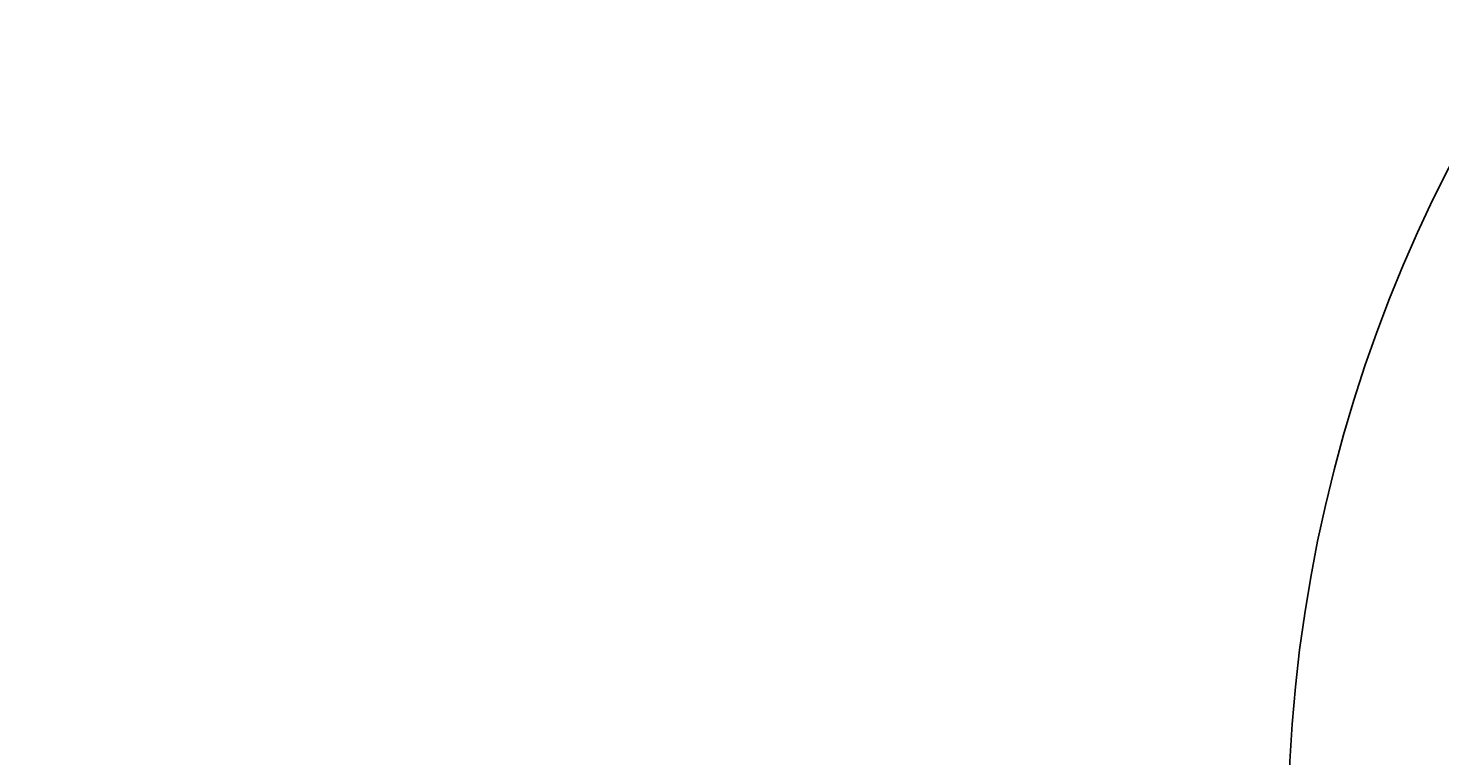
# Model space of a CAD drawing. Units: inches. Extents: x 1998 to 2588, y 1139 to 1977.
# Tile 67 of 134: x 2160 to 2192, y 1762 to 1779. Entities that reach past the tile are written whole.
import ezdxf

# ---------------------------------------------------------------- set-up
doc = ezdxf.new("R2010")
doc.units = ezdxf.units.IN
doc.layers.add('A-ANNO-DIMS', color=2, linetype='Continuous', lineweight=18)
doc.layers.add('DOOR', color=52, linetype='Continuous', lineweight=25)
doc.styles.get("Standard").update_dxf_attribs({"font": 'arial.ttf'})
doc.dimstyles.get("Standard").update_dxf_attribs({"dimtxt": 0.18, "dimasz": 0.18, "dimexe": 0.18, "dimexo": 0.0625, "dimgap": 0.09, "dimtad": 0, "dimtih": 1, "dimtoh": 1, "dimdec": 4, "dimzin": 0, "dimdsep": 46, "dimtxsty": 'Standard', "dimcen": 0.09, "dimadec": 0, "dimazin": 0, "dimtfac": 1, "dimtdec": 4, "dimtofl": 0, "dimtmove": 0, "dimatfit": 3, "dimfxl": 1, "dimtolj": 1, "dimtzin": 0, "dimarcsym": 0})

# ---------------------------------------------------------------- blocks, each defined once
blk = doc.blocks.new('*U2')
blk.add_arc((0, 0), 40, 0, 90)
blk = doc.blocks.new('*D37')
at = {"layer": 'A-ANNO-DIMS', "color": 0, "lineweight": -2, "transparency": 16777216}
for p, q in [((2148.455, 1612.795), (2148.455, 1977.362)), ((2197.45, 1612.795), (2197.45, 1977.362)), ((2148.635, 1977.182), (2172.73, 1977.182)), ((2197.27, 1977.182), (2173.175, 1977.182))]:
    blk.add_line(p, q, dxfattribs=at)
at = {"layer": 'A-ANNO-DIMS', "color": 0, "transparency": 16777216}
for points in [[(2148.635, 1977.212), (2148.635, 1977.152), (2148.455, 1977.182)], [(2197.27, 1977.212), (2197.27, 1977.152), (2197.45, 1977.182)]]:
    blk.add_solid(points, dxfattribs=at)
at = {"layer": 'Defpoints', "color": 0, "transparency": 16777216}
for p in [(2197.45, 1977.182), (2148.455, 1612.732), (2197.45, 1612.732)]:
    blk.add_point(p, dxfattribs=at)
at = {"layer": 'A-ANNO-DIMS', "color": 0, "transparency": 16777216, "insert": (2172.952, 1977.182), "char_height": 0.18, "attachment_point": 5}
blk.add_mtext('\\A1;49', dxfattribs=at)

msp = doc.modelspace()

# ---------------------------------------------------------------- block references
at = {"layer": 'DOOR', "xscale": -0.8354643497673233, "yscale": 0.8354643497673233, "zscale": 0.8354643497673233}
msp.add_blockref('*U2', (2221.7204, 1760.2452), dxfattribs=at)

# ---------------------------------------------------------------- dimensions: what is measured, and where the dimension line sits
at = {"layer": 'A-ANNO-DIMS'}
dim = msp.add_linear_dim(base=(2197.4499, 1977.1824), p1=(2148.4548, 1612.7324), p2=(2197.4499, 1612.7324), dimstyle='Standard', override={"dimdec": 0, "dimlfac": 1, "dimrnd": 0, "dimzin": 0, "dimdsep": 46, "dimlunit": 2}, dxfattribs=at)
dim.commit()
dim.dimension.update_dxf_attribs({"geometry": '*D37', "text_midpoint": (2172.9524, 1977.1824)})

doc.saveas('drawing.dxf')
